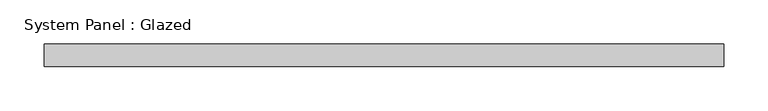
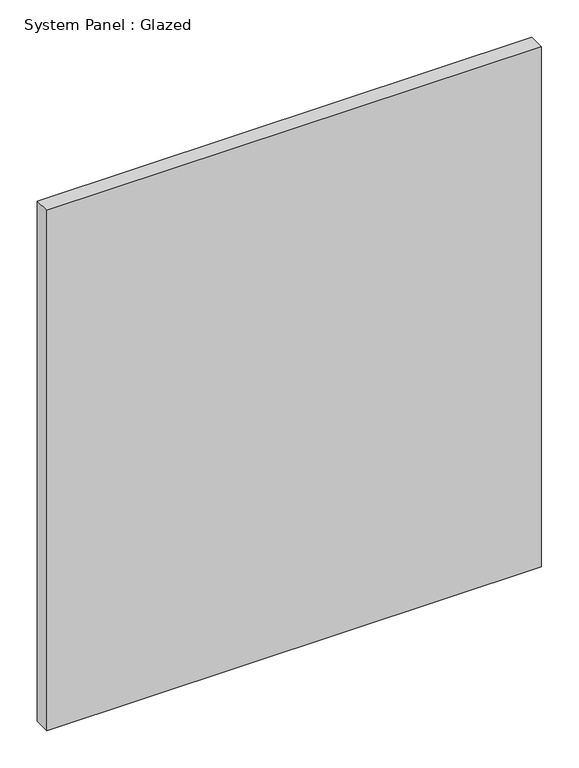
"""IFC4 building model written with IfcOpenShell, lengths in millimetres: plate geometry, System Panel : Glazed."""

from ifc_helpers import new_model, si_unit, origin, origin_with_axes, place, context, project, spatial, polyline, outline, extrude, source, transform, mapped, element, save


def system_panel_glazed_6813505b(model_context):
    return source(origin(), model_context, "Body", "SweptSolid", [
        extrude(outline(polyline([(383.50825, 19.05), (-383.50825, 19.05), (-383.50825, 44.45), (383.50825, 44.45), (383.50825, 19.05)])), origin_with_axes(), (0.0, 0.0, 1.0), 852.7415),
    ])


if __name__ == "__main__":
    model = new_model("IFC4")
    model_context = context("Model", 3, world=origin())
    ifc_project = project(units=[si_unit("LENGTHUNIT", "METRE", prefix="MILLI")], contexts=[model_context])
    site = spatial("IfcSite", under=ifc_project)
    building = spatial("IfcBuilding", under=site)
    placement = place(None, origin())
    system_panel_glazed_shape = system_panel_glazed_6813505b(model_context)
    element("IfcPlate", 1, ObjectType="System Panel : Glazed", at=placement, inside=building, context=model_context, shape_type="MappedRepresentation", body=[
        mapped(system_panel_glazed_shape, transform((0.0, 0.0, 0.0), x_axis=(1.0, 0.0, 0.0), y_axis=(0.0, 1.0, 0.0), z_axis=(0.0, 0.0, 1.0))),
    ])
    save(model, "model.ifc")

# Revit data of these elements
# Type "System Panel : Glazed"
#   Construction Type Id = "GSP4R"
#   Analytic Construction = "1/8 in Pilkington single glazing"
#   Visual Light Transmittance = 0.9
#   Solar Heat Gain Coefficient = 0.86
#   Heat Transfer Coefficient (U) = 1.18115 BTU/(h·ft²·°F)
#   Define Thermal Properties by = 1
# Element 1 (IfcPlate, "System Panel : Glazed")
#   Materials on its faces: "Glass"
# Materials
#   "Glass": class "Glass", colour RGB 0 128 192, transparency 0.75, Description = "Soda Lime Glass", Cost = 0
